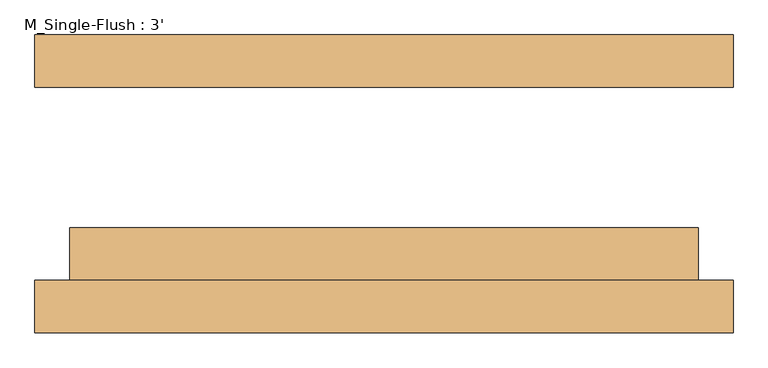
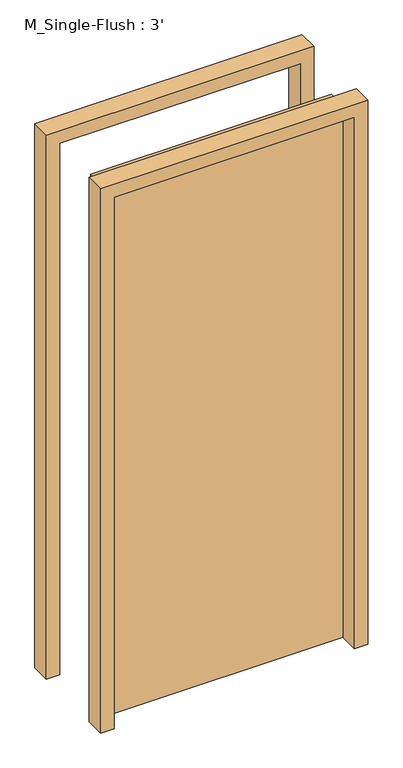
"""IFC4 building model written with IfcOpenShell, lengths in millimetres: door geometry, M_Single-Flush : 3'."""

from ifc_helpers import new_model, si_unit, frame, origin, origin_with_axes, place, context, project, spatial, polyline, outline, extrude, source, transform, mapped, element, save


def m_single_flush_3_bd8c2fc5(model_context):
    return source(origin(), model_context, "Body", "SweptSolid", [
        extrude(outline(polyline([(2184.4, -508.0), (0.0, -508.0), (0.0, -457.2), (2133.6, -457.2), (2133.6, 457.2), (0.0, 457.2), (0.0, 508.0), (2184.4, 508.0), (2184.4, -508.0)])), frame((0.0, -216.6, 0.0), z_axis=(0.0, 1.0, 0.0), x_axis=(0.0, 0.0, 1.0)), (0.0, 0.0, 1.0), 76.2),
        extrude(outline(polyline([(2184.4, 508.0), (2184.4, -508.0), (0.0, -508.0), (0.0, -457.2), (2133.6, -457.2), (2133.6, 457.2), (0.0, 457.2), (0.0, 508.0), (2184.4, 508.0)])), frame((0.0, 140.4, 0.0), z_axis=(0.0, 1.0, 0.0), x_axis=(0.0, 0.0, 1.0)), (0.0, 0.0, 1.0), 76.2),
        extrude(outline(polyline([(457.2, -64.2), (457.2, -140.4), (-457.2, -140.4), (-457.2, -64.2), (457.2, -64.2)])), origin_with_axes(), (0.0, 0.0, 1.0), 2133.6),
    ])


if __name__ == "__main__":
    model = new_model("IFC4")
    model_context = context("Model", 3, world=origin())
    ifc_project = project(units=[si_unit("LENGTHUNIT", "METRE", prefix="MILLI")], contexts=[model_context])
    site = spatial("IfcSite", under=ifc_project)
    building = spatial("IfcBuilding", under=site)
    placement = place(None, origin())
    m_single_flush_3_shape = m_single_flush_3_bd8c2fc5(model_context)
    element("IfcDoor", 1, ObjectType="M_Single-Flush : 3'", at=placement, inside=building, context=model_context, shape_type="MappedRepresentation", body=[
        mapped(m_single_flush_3_shape, transform((0.0, 0.0, 0.0), x_axis=(1.0, 0.0, 0.0), y_axis=(0.0, 1.0, 0.0), z_axis=(0.0, 0.0, 1.0))),
    ])
    save(model, "model.ifc")

# Revit data of these elements
# Type "M_Single-Flush : 3'"
#   Type Mark = "23"
#   Thickness = 0' - 3"
#   Height = 7' - 0"
#   Trim Projection Ext = 0' - 3"
#   Trim Projection Int = 0' - 3"
#   Trim Width = 0' - 2"
#   Width = 3' - 0"
#   Wall Closure = 2
#   Door Material = Door - Panel
#   Frame Material = Door - Panel
#   Function = (empty or 0)
# Element 1 (IfcDoor, "M_Single-Flush : 3'")
#   Materials on its faces: "Door - Panel"
# Materials
#   "Door - Panel": class "Wood", colour RGB 114 82 51, transparency 0
